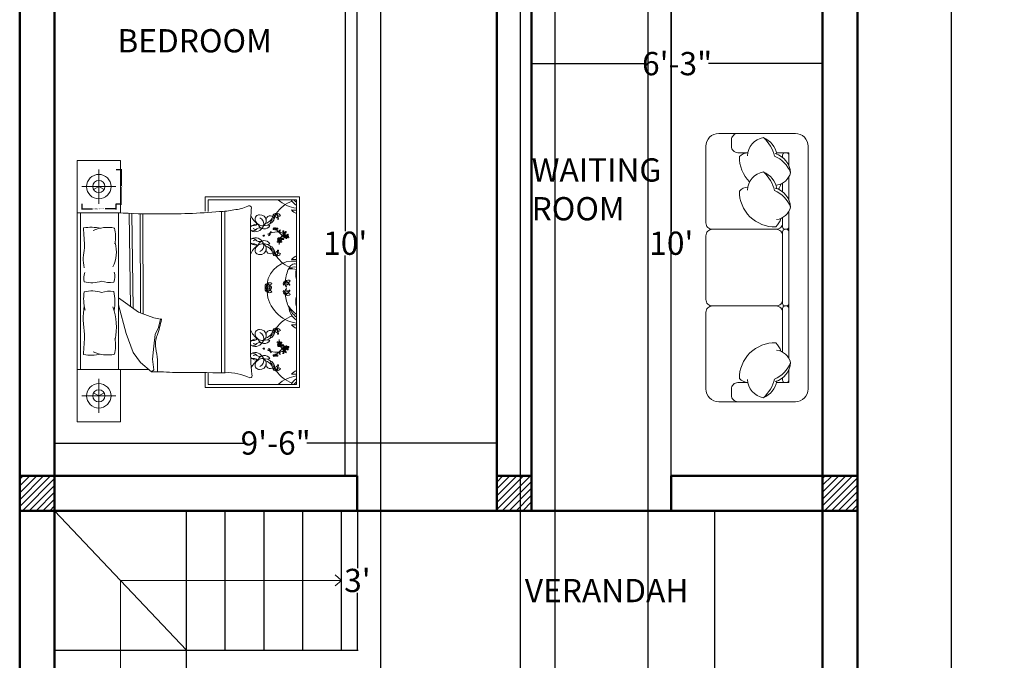
# Model space of a CAD drawing. Units: inches. Extents: x 0 to 281, y -535 to 46.
# Tile 2 of 22: x 27 to 281, y -440 to -275. Entities that reach past the tile are written whole.
import ezdxf

# ---------------------------------------------------------------- set-up
doc = ezdxf.new("R2010")
doc.units = ezdxf.units.IN
doc.header["$MEASUREMENT"] = 0
for name, color, linetype, lineweight in [('A-ANNO-DIMS', 2, 'Continuous', 18), ('A-ANNO-SYMB', 2, 'Continuous', 18), ('A-AREA-IDEN', 7, 'Continuous', 25), ('A-COLS', 7, 'Continuous', 50), ('A-COLS-PATT', 152, 'Continuous', 13), ('A-FLOR-STRS', 7, 'Continuous', 25), ('A-FURN', 8, 'Continuous', 18), ('A-WALL', 7, 'Continuous', 50)]:
    doc.layers.add(name, color=color, linetype=linetype, lineweight=lineweight)
doc.styles.get("Standard").update_dxf_attribs({"font": 'arial.ttf'})
doc.dimstyles.get("Standard").update_dxf_attribs({"dimtxt": 0.18, "dimasz": 0.18, "dimexe": 0.18, "dimexo": 0.0625, "dimgap": 0.09, "dimtad": 0, "dimtih": 1, "dimtoh": 1, "dimdec": 0, "dimzin": 0, "dimdsep": 46, "dimlunit": 3, "dimtxsty": 'Standard', "dimcen": 0.09, "dimadec": 0, "dimazin": 0, "dimtfac": 1, "dimtdec": 0, "dimtofl": 0, "dimtmove": 0, "dimatfit": 3, "dimfxl": 1, "dimtolj": 1, "dimtzin": 0, "dimarcsym": 0})

# ---------------------------------------------------------------- blocks, each defined once
blk = doc.blocks.new('*D9')
at = {"layer": 'A-ANNO-DIMS', "color": 0, "lineweight": -2, "transparency": 16777216}
for p, q in [((114.4, -272.41), (111.21, -272.41)), ((111.39, -272.59), (111.39, -329.26)), ((111.39, -392.23), (111.39, -335.56)), ((114.4, -392.41), (111.21, -392.41))]:
    blk.add_line(p, q, dxfattribs=at)
at = {"layer": 'A-ANNO-DIMS', "color": 0, "transparency": 16777216}
for points in [[(111.36, -272.59), (111.42, -272.59), (111.39, -272.41)], [(111.36, -392.23), (111.42, -392.23), (111.39, -392.41)]]:
    blk.add_solid(points, dxfattribs=at)
at = {"layer": 'Defpoints', "color": 0, "transparency": 16777216}
for p in [(111.39, -272.41), (114.46, -272.41), (114.46, -392.41)]:
    blk.add_point(p, dxfattribs=at)
at = {"layer": 'A-ANNO-DIMS', "color": 0, "transparency": 16777216, "insert": (111.39, -332.41), "char_height": 6, "attachment_point": 5}
blk.add_mtext("\\A1;10'", dxfattribs=at)
blk = doc.blocks.new('*D10')
at = {"layer": 'A-ANNO-DIMS', "color": 0, "lineweight": -2, "transparency": 16777216}
for p, q in [((36.46, -383.89), (36.46, -383.77)), ((36.64, -383.95), (85.39, -383.95)), ((150.28, -383.95), (101.52, -383.95)), ((150.46, -383.89), (150.46, -383.77))]:
    blk.add_line(p, q, dxfattribs=at)
at = {"layer": 'A-ANNO-DIMS', "color": 0, "transparency": 16777216}
for points in [[(36.64, -383.92), (36.64, -383.98), (36.46, -383.95)], [(150.28, -383.92), (150.28, -383.98), (150.46, -383.95)]]:
    blk.add_solid(points, dxfattribs=at)
at = {"layer": 'Defpoints', "color": 0, "transparency": 16777216}
for p in [(36.46, -383.95), (150.46, -383.95), (150.46, -383.95)]:
    blk.add_point(p, dxfattribs=at)
at = {"layer": 'A-ANNO-DIMS', "color": 0, "transparency": 16777216, "insert": (93.46, -383.95), "char_height": 6, "attachment_point": 5}
blk.add_mtext('\\A1;9\'-6"', dxfattribs=at)
blk = doc.blocks.new('*D11')
at = {"layer": 'A-ANNO-DIMS', "color": 0, "lineweight": -2, "transparency": 16777216}
for p, q in [((159.46, -286.02), (159.46, -285.9)), ((159.64, -286.08), (188.88, -286.08)), ((234.28, -286.08), (205.04, -286.08)), ((234.46, -286.02), (234.46, -285.9))]:
    blk.add_line(p, q, dxfattribs=at)
at = {"layer": 'A-ANNO-DIMS', "color": 0, "transparency": 16777216}
for points in [[(159.64, -286.05), (159.64, -286.11), (159.46, -286.08)], [(234.28, -286.05), (234.28, -286.11), (234.46, -286.08)]]:
    blk.add_solid(points, dxfattribs=at)
at = {"layer": 'Defpoints', "color": 0, "transparency": 16777216}
for p in [(159.46, -286.08), (234.46, -286.08), (234.46, -286.08)]:
    blk.add_point(p, dxfattribs=at)
at = {"layer": 'A-ANNO-DIMS', "color": 0, "transparency": 16777216, "insert": (196.96, -286.08), "char_height": 6, "attachment_point": 5}
blk.add_mtext('\\A1;6\'-3"', dxfattribs=at)
blk = doc.blocks.new('*D12')
at = {"layer": 'A-ANNO-DIMS', "color": 0, "lineweight": -2, "transparency": 16777216}
for p, q in [((195.46, -272.59), (195.46, -329.26)), ((195.52, -272.41), (195.64, -272.41)), ((195.46, -392.23), (195.46, -335.56)), ((195.52, -392.41), (195.64, -392.41))]:
    blk.add_line(p, q, dxfattribs=at)
at = {"layer": 'A-ANNO-DIMS', "color": 0, "transparency": 16777216}
for points in [[(195.43, -272.59), (195.49, -272.59), (195.46, -272.41)], [(195.43, -392.23), (195.49, -392.23), (195.46, -392.41)]]:
    blk.add_solid(points, dxfattribs=at)
at = {"layer": 'Defpoints', "color": 0, "transparency": 16777216}
for p in [(195.46, -272.41), (195.46, -392.41), (195.46, -392.41)]:
    blk.add_point(p, dxfattribs=at)
at = {"layer": 'A-ANNO-DIMS', "color": 0, "transparency": 16777216, "insert": (195.46, -332.41), "char_height": 6, "attachment_point": 5}
blk.add_mtext("\\A1;10'", dxfattribs=at)
blk = doc.blocks.new('*D13')
at = {"layer": 'A-ANNO-DIMS', "color": 0, "lineweight": -2, "transparency": 16777216}
for p, q in [((206.57, -401.59), (206.57, -446.76)), ((206.63, -401.41), (206.75, -401.41)), ((206.57, -498.23), (206.57, -453.06)), ((206.63, -498.41), (206.75, -498.41))]:
    blk.add_line(p, q, dxfattribs=at)
at = {"layer": 'A-ANNO-DIMS', "color": 0, "transparency": 16777216}
for points in [[(206.54, -401.59), (206.6, -401.59), (206.57, -401.41)], [(206.54, -498.23), (206.6, -498.23), (206.57, -498.41)]]:
    blk.add_solid(points, dxfattribs=at)
at = {"layer": 'Defpoints', "color": 0, "transparency": 16777216}
for p in [(206.57, -401.41), (206.57, -498.41), (206.57, -498.41)]:
    blk.add_point(p, dxfattribs=at)
at = {"layer": 'A-ANNO-DIMS', "color": 0, "transparency": 16777216, "insert": (206.57, -449.91), "char_height": 6, "attachment_point": 5}
blk.add_mtext('\\A1;8\'-1"', dxfattribs=at)
blk = doc.blocks.new('*D15')
at = {"layer": 'A-ANNO-DIMS', "color": 0, "lineweight": -2, "transparency": 16777216}
for p, q in [((110.52, -401.41), (114.71, -401.41)), ((114.53, -401.59), (114.53, -416.26)), ((114.53, -437.23), (114.53, -422.57)), ((110.52, -437.41), (114.71, -437.41))]:
    blk.add_line(p, q, dxfattribs=at)
at = {"layer": 'A-ANNO-DIMS', "color": 0, "transparency": 16777216}
for points in [[(114.5, -401.59), (114.56, -401.59), (114.53, -401.41)], [(114.5, -437.23), (114.56, -437.23), (114.53, -437.41)]]:
    blk.add_solid(points, dxfattribs=at)
at = {"layer": 'Defpoints', "color": 0, "transparency": 16777216}
for p in [(110.46, -401.41), (110.46, -437.41), (114.53, -437.41)]:
    blk.add_point(p, dxfattribs=at)
at = {"layer": 'A-ANNO-DIMS', "color": 0, "transparency": 16777216, "insert": (114.53, -419.41), "char_height": 6, "attachment_point": 5}
blk.add_mtext("\\A1;3'", dxfattribs=at)
blk = doc.blocks.new('*D18')
at = {"layer": 'A-ANNO-DIMS', "color": 0, "lineweight": -2, "transparency": 16777216}
for p, q in [((243.52, 18.59), (267.93, 18.59)), ((267.75, 18.41), (267.75, -241.26)), ((267.75, -507.23), (267.75, -247.57)), ((243.52, -507.41), (267.93, -507.41))]:
    blk.add_line(p, q, dxfattribs=at)
at = {"layer": 'A-ANNO-DIMS', "color": 0, "transparency": 16777216}
for points in [[(267.72, 18.41), (267.78, 18.41), (267.75, 18.59)], [(267.72, -507.23), (267.78, -507.23), (267.75, -507.41)]]:
    blk.add_solid(points, dxfattribs=at)
at = {"layer": 'Defpoints', "color": 0, "transparency": 16777216}
for p in [(243.46, 18.59), (243.46, -507.41), (267.75, -507.41)]:
    blk.add_point(p, dxfattribs=at)
at = {"layer": 'A-ANNO-DIMS', "color": 0, "transparency": 16777216, "insert": (267.75, -244.41), "char_height": 6, "attachment_point": 5}
blk.add_mtext('\\A1;43\'-10"', dxfattribs=at)
blk = doc.blocks.new('BEDSIDE-LAMP-SMALL')
for p, q in [((4.41, 0), (4.41, 8.82)), ((8.82, 4.41), (0, 4.41))]:
    blk.add_line(p, q)
for points in [[(4.41, 4.41), (3.04, 3.62)], [(4.41, 4.41), (5.77, 3.62)]]:
    blk.add_lwpolyline(points)
for radius in [3.15, 1.57]:
    blk.add_circle((4.41, 4.41), radius)
blk = doc.blocks.new('SOFA-THROW-PILLOW')
for points in [[(11.04, 3.89, 0.165541), (13.21, 4.91, 0.425989), (3.78, 14.16, 0.121523), (2.47, 11.97, -7.115464)], [(3.93, 4.15, -0.306663), (0, 9.06, -0.30633), (3.59, 12.27, 0.872847)], [(6.98, 0, -0.14773), (4.15, 4.82, -0.213343), (0, 9.06, -0.178662)], [(11.14, 4.72, -0.356772), (6.98, 0, -0.249542), (3.56, 4.28, 9.61688)]]:
    blk.add_lwpolyline(points, format="xyb")
blk = doc.blocks.new('*D38')
at = {"layer": 'A-ANNO-DIMS', "color": 0, "lineweight": -2, "transparency": 16777216}
for p, q in [((43.45, -322.28), (43.45, -323.72)), ((52.27, -322.28), (52.27, -323.72)), ((43.63, -323.54), (46.26, -323.54)), ((52.09, -323.54), (49.46, -323.54))]:
    blk.add_line(p, q, dxfattribs=at)
at = {"layer": 'A-ANNO-DIMS', "color": 0, "transparency": 16777216}
for points in [[(43.63, -323.51), (43.63, -323.57), (43.45, -323.54)], [(52.09, -323.51), (52.09, -323.57), (52.27, -323.54)]]:
    blk.add_solid(points, dxfattribs=at)
at = {"layer": 'Defpoints', "color": 0, "transparency": 16777216}
for p in [(43.45, -322.21), (52.27, -322.21), (52.27, -323.54)]:
    blk.add_point(p, dxfattribs=at)
at = {"layer": 'A-ANNO-DIMS', "color": 0, "transparency": 16777216, "insert": (47.86, -323.54), "char_height": 0.18, "attachment_point": 5}
blk.add_mtext('\\A1;BEDSIDE LAMP 0\'-9" TYP.', dxfattribs=at)
blk = doc.blocks.new('*D39')
at = {"layer": 'A-ANNO-DIMS', "color": 0, "lineweight": -2, "transparency": 16777216}
for p, q in [((52.33, -313.4), (53.77, -313.4)), ((53.59, -313.58), (53.59, -317.63)), ((53.59, -322.03), (53.59, -317.99)), ((52.33, -322.21), (53.77, -322.21))]:
    blk.add_line(p, q, dxfattribs=at)
at = {"layer": 'A-ANNO-DIMS', "color": 0, "transparency": 16777216}
for points in [[(53.56, -313.58), (53.62, -313.58), (53.59, -313.4)], [(53.56, -322.03), (53.62, -322.03), (53.59, -322.21)]]:
    blk.add_solid(points, dxfattribs=at)
at = {"layer": 'Defpoints', "color": 0, "transparency": 16777216}
for p in [(52.27, -313.4), (53.59, -313.4), (52.27, -322.21)]:
    blk.add_point(p, dxfattribs=at)
at = {"layer": 'A-ANNO-DIMS', "color": 0, "transparency": 16777216, "insert": (53.59, -317.81), "char_height": 0.18, "attachment_point": 5}
blk.add_mtext('\\A1;0\'-9" TYP.', dxfattribs=at)
blk = doc.blocks.new('*D41')
at = {"layer": 'A-ANNO-DIMS', "color": 0, "lineweight": -2, "transparency": 16777216}
for p, q in [((120.46, -131.47), (120.46, -535.04)), ((156.46, -131.47), (156.46, -535.04)), ((120.64, -534.86), (138.13, -534.86)), ((156.28, -534.86), (138.79, -534.86))]:
    blk.add_line(p, q, dxfattribs=at)
at = {"layer": 'A-ANNO-DIMS', "color": 0, "transparency": 16777216}
for points in [[(120.64, -534.83), (120.64, -534.89), (120.46, -534.86)], [(156.28, -534.83), (156.28, -534.89), (156.46, -534.86)]]:
    blk.add_solid(points, dxfattribs=at)
at = {"layer": 'Defpoints', "color": 0, "transparency": 16777216}
for p in [(120.46, -131.41), (156.46, -131.41), (156.46, -534.86)]:
    blk.add_point(p, dxfattribs=at)
at = {"layer": 'A-ANNO-DIMS', "color": 0, "transparency": 16777216, "insert": (138.46, -534.86), "char_height": 0.18, "attachment_point": 5}
blk.add_mtext('\\A1;3\'-0"', dxfattribs=at)
blk = doc.blocks.new('*D42')
at = {"layer": 'A-ANNO-DIMS', "color": 0, "lineweight": -2, "transparency": 16777216}
for p, q in [((165.46, -131.47), (165.46, -535.04)), ((189.46, -131.47), (189.46, -535.04)), ((165.64, -534.86), (177.13, -534.86)), ((189.28, -534.86), (177.79, -534.86))]:
    blk.add_line(p, q, dxfattribs=at)
at = {"layer": 'A-ANNO-DIMS', "color": 0, "transparency": 16777216}
for points in [[(165.64, -534.83), (165.64, -534.89), (165.46, -534.86)], [(189.28, -534.83), (189.28, -534.89), (189.46, -534.86)]]:
    blk.add_solid(points, dxfattribs=at)
at = {"layer": 'Defpoints', "color": 0, "transparency": 16777216}
for p in [(165.46, -131.41), (189.46, -131.41), (189.46, -534.86)]:
    blk.add_point(p, dxfattribs=at)
at = {"layer": 'A-ANNO-DIMS', "color": 0, "transparency": 16777216, "insert": (177.46, -534.86), "char_height": 0.18, "attachment_point": 5}
blk.add_mtext('\\A1;2\'-0"', dxfattribs=at)
blk = doc.blocks.new('*D47')
at = {"layer": 'A-ANNO-DIMS', "color": 0, "lineweight": -2, "transparency": 16777216}
for p, q in [((114.46, -392.35), (114.46, 46.22)), ((114.64, 46.04), (132.13, 46.04)), ((150.28, 46.04), (132.79, 46.04)), ((150.46, -392.35), (150.46, 46.22))]:
    blk.add_line(p, q, dxfattribs=at)
at = {"layer": 'A-ANNO-DIMS', "color": 0, "transparency": 16777216}
for points in [[(114.64, 46.07), (114.64, 46.01), (114.46, 46.04)], [(150.28, 46.07), (150.28, 46.01), (150.46, 46.04)]]:
    blk.add_solid(points, dxfattribs=at)
at = {"layer": 'Defpoints', "color": 0, "transparency": 16777216}
for p in [(150.46, 46.04), (114.46, -392.41), (150.46, -392.41)]:
    blk.add_point(p, dxfattribs=at)
at = {"layer": 'A-ANNO-DIMS', "color": 0, "transparency": 16777216, "insert": (132.46, 46.04), "char_height": 0.18, "attachment_point": 5}
blk.add_mtext('\\A1;3\'-0"', dxfattribs=at)
blk = doc.blocks.new('*D48')
at = {"layer": 'A-ANNO-DIMS', "color": 0, "lineweight": -2, "transparency": 16777216}
for p, q in [((159.46, -392.35), (159.46, 46.22)), ((159.64, 46.04), (177.13, 46.04)), ((195.28, 46.04), (177.79, 46.04)), ((195.46, -392.35), (195.46, 46.22))]:
    blk.add_line(p, q, dxfattribs=at)
at = {"layer": 'A-ANNO-DIMS', "color": 0, "transparency": 16777216}
for points in [[(159.64, 46.07), (159.64, 46.01), (159.46, 46.04)], [(195.28, 46.07), (195.28, 46.01), (195.46, 46.04)]]:
    blk.add_solid(points, dxfattribs=at)
at = {"layer": 'Defpoints', "color": 0, "transparency": 16777216}
for p in [(195.46, 46.04), (159.46, -392.41), (195.46, -392.41)]:
    blk.add_point(p, dxfattribs=at)
at = {"layer": 'A-ANNO-DIMS', "color": 0, "transparency": 16777216, "insert": (177.46, 46.04), "char_height": 0.18, "attachment_point": 5}
blk.add_mtext('\\A1;3\'-0"', dxfattribs=at)

msp = doc.modelspace()

# ---------------------------------------------------------------- hatches: boundary and pattern name
at = {"layer": 'A-COLS-PATT'}
h = msp.add_hatch(dxfattribs=at)
h.set_pattern_fill('ANSI31', color=256, scale=10)
h.paths.add_polyline_path([(36.46, 18.59), (27.46, 18.59), (27.46, 9.59), (36.46, 9.59)])
h.paths.add_polyline_path([(165.46, 18.59), (156.46, 18.59), (156.46, 9.59), (165.46, 9.59)])
h.paths.add_polyline_path([(243.46, 18.59), (234.46, 18.59), (234.46, 9.59), (243.46, 9.59)])
h.paths.add_polyline_path([(243.46, -122.41), (234.46, -122.41), (234.46, -131.41), (243.46, -131.41)])
h.paths.add_polyline_path([(36.46, -122.41), (27.46, -122.41), (27.46, -131.41), (36.46, -131.41)])
h.paths.add_polyline_path([(36.46, -498.41), (27.46, -498.41), (27.46, -507.41), (36.46, -507.41)])
h.paths.add_polyline_path([(243.46, -498.41), (234.46, -498.41), (234.46, -507.41), (243.46, -507.41)])
h.paths.add_polyline_path([(159.46, -498.41), (150.46, -498.41), (150.46, -507.41), (159.46, -507.41)])
h.paths.add_polyline_path([(36.46, -392.41), (27.46, -392.41), (27.46, -401.41), (36.46, -401.41)])
h.paths.add_polyline_path([(159.46, -392.41), (150.46, -392.41), (150.46, -401.41), (159.46, -401.41)])
h.paths.add_polyline_path([(243.46, -392.41), (234.46, -392.41), (234.46, -401.41), (243.46, -401.41)])
h.paths.add_polyline_path([(36.46, -263.41), (27.46, -263.41), (27.46, -272.41), (36.46, -272.41)])
h.paths.add_polyline_path([(243.46, -263.41), (234.46, -263.41), (234.46, -272.41), (243.46, -272.41)])

# ---------------------------------------------------------------- linework, layer by layer
at = {"layer": 'A-ANNO-SYMB'}
for p, q in [((110.46, -419.41), (108.77, -418)), ((110.46, -419.41), (53.46, -419.41)), ((53.46, -419.41), (53.46, -480.41)), ((110.46, -419.41), (108.77, -420.82))]:
    msp.add_line(p, q, dxfattribs=at)
at = {"layer": 'A-COLS'}
msp.add_line((150.46, -392.41), (159.46, -392.41), dxfattribs=at)
at = {"layer": 'A-FLOR-STRS'}
for p, q in [((70.46, -437.41), (36.46, -401.41)), ((70.46, -498.41), (70.46, -401.41)), ((80.46, -437.41), (80.46, -401.41)), ((90.46, -437.41), (90.46, -401.41)), ((100.46, -437.41), (100.46, -401.41)), ((110.46, -437.41), (110.46, -401.41)), ((36.46, -437.41), (110.46, -437.41))]:
    msp.add_line(p, q, dxfattribs=at)
at = {"layer": 'A-FURN'}
for p, q in [((42.24, -378.52), (42.24, -311.06)), ((75.31, -324.18), (75.31, -320.44)), ((75.31, -320.44), (99.61, -320.44)), ((76.09, -321.22), (76.09, -324.19)), ((98.83, -321.22), (76.09, -321.22)), ((98.83, -368.84), (98.83, -321.22)), ((99.61, -320.44), (99.61, -369.62)), ((43.11, -324.55), (43.11, -365.03)), ((52.9, -365.03), (52.9, -324.55)), ((55.7, -324.73), (56.04, -348.75)), ((56.39, -324.76), (56.74, -349.26)), ((58.52, -324.8), (58.62, -350.41)), ((59.21, -324.79), (59.32, -350.68)), ((79.52, -324.25), (79.52, -365.81)), ((80.36, -324.18), (80.36, -365.81)), ((91.99, -327.87), (91.23, -327.72)), ((86.98, -331.1), (86.98, -358.49)), ((91.99, -332.58), (91.23, -332.73)), ((52.9, -346.5), (58.05, -350.19)), ((54.9, -355.66), (52.9, -348.3)), ((58.05, -350.19), (62.01, -351.7)), ((62.01, -351.7), (63.78, -351.97)), ((63.78, -351.97), (63.23, -354.16)), ((63.23, -354.16), (62.41, -355.93)), ((56.68, -360.58), (54.9, -355.66)), ((62.41, -355.93), (62.01, -358.94)), ((91.99, -357.47), (91.23, -357.32)), ((62.01, -358.94), (61.73, -362.35)), ((58.59, -363.17), (56.68, -360.58)), ((61.73, -362.35), (62.01, -365.09)), ((91.99, -362.19), (91.23, -362.34)), ((42.24, -365.03), (60.75, -365.03)), ((61.46, -365.63), (58.59, -363.17)), ((62.01, -365.09), (61.46, -365.63)), ((75.31, -369.62), (75.31, -365.8)), ((76.09, -365.8), (76.09, -368.84)), ((99.61, -369.62), (75.31, -369.62)), ((76.09, -368.84), (98.83, -368.84))]:
    msp.add_line(p, q, dxfattribs=at)
at = {"layer": 'A-FURN', "ltscale": 0.03}
msp.add_lwpolyline([(207.69, -373.3, -0.414214), (204.39, -370.01), (204.39, -350.24, -0.414214), (206.04, -348.59, -0.414214), (204.39, -346.94), (204.39, -330.47, -0.414214), (206.04, -328.82, -0.414214), (204.39, -327.17), (204.39, -307.4, -0.414214), (207.69, -304.11), (227.46, -304.11, -0.414214), (230.75, -307.4), (230.75, -370.01, -0.414214), (227.46, -373.3)], format="xyb", close=True, dxfattribs=at)
at = {"layer": 'A-FURN'}
for points in [[(215.18, -309.05), (212.63, -309.05, -0.414214), (210.98, -307.4), (210.98, -305.75, -0.414214), (212.63, -304.11)], [(215.08, -309.88, -0.356772), (219.24, -305.15, -0.249542), (222.66, -309.43, 9.61688)], [(219.24, -305.15, -0.14773), (222.07, -309.97, -0.213343), (226.22, -314.22, -0.178662)], [(215.18, -309.05, 0.165541), (213.01, -310.06, 0.200231), (215.66, -316.6, 0.121523)], [(222.29, -309.3, -0.306663), (226.22, -314.22, -0.30633), (222.63, -317.43, 0.872847)], [(225.81, -312.51), (225.81, -309.05), (222.57, -309.05, -0.414214)], [(224.16, -310.31), (224.16, -309.71, -0.414214), (224.82, -309.05), (225.15, -309.05, -0.414214), (225.81, -309.71)], [(225.81, -309.71), (225.81, -312.51, -0.414214)], [(223.1, -318.5, 0.071865), (223.75, -317.12, -7.115464)], [(224.16, -319.18), (224.16, -316.91, -0.414214)], [(225.81, -315.26), (225.81, -321.39, -0.414214)], [(78.98, -324.27, 0.056112), (82.7, -323.78, 0.095341), (86.27, -322.83)], [(225.81, -324.13), (225.81, -328.16, -0.414214), (225.15, -328.82), (224.82, -328.82, -0.414214), (224.16, -328.16), (224.16, -325.79, -0.414214)], [(224.16, -327.17, -0.414214), (222.52, -328.82), (206.04, -328.82, -0.414214)], [(43.92, -328.43, -0.074897), (48.33, -328.51, 0.472817)], [(224.16, -330.47, 0.414214), (222.52, -328.82)], [(48.57, -342.23, -0.14099), (44.08, -342.36, -0.235245)], [(48.57, -345.11, 0.14099), (44.08, -344.97, 0.235245)], [(224.16, -346.94, -0.414214), (222.52, -348.59)], [(224.16, -350.24, 0.414214), (222.52, -348.59), (206.04, -348.59, 0.414214)], [(225.81, -362.15), (225.81, -349.25, 0.414214), (225.15, -348.59), (224.82, -348.59, 0.414214), (224.16, -349.25), (224.16, -360.5, 0.414214)], [(43.92, -361.15, 0.074897), (48.33, -361.07, -0.472817)], [(225.81, -367.7), (225.81, -364.9, 0.414214)], [(67.64, -365.77, 0.001242), (80.44, -365.81, -0.127202), (86.81, -367.16)], [(224.16, -367.1), (224.16, -367.7, 0.414214), (224.82, -368.36), (225.15, -368.36, 0.414214), (225.81, -367.7)], [(212.63, -373.3, -0.414214), (210.98, -371.66), (210.98, -370.01, -0.414214), (212.63, -368.36), (215.18, -368.36)]]:
    msp.add_lwpolyline(points, format="xyb", dxfattribs=at)
for points in [[(42.24, -324.55), (53.48, -324.55), (53.48, -311.06), (42.24, -311.06)], [(225.81, -321.39), (225.81, -315.26)], [(225.81, -362.15), (225.81, -324.13)], [(53.48, -365.03), (53.48, -378.52), (42.24, -378.52)], [(222.57, -368.36), (225.81, -368.36), (225.81, -364.9)]]:
    msp.add_lwpolyline(points, dxfattribs=at)
msp.add_lwpolyline([(225.81, -329.48), (225.81, -347.93, -0.414214), (225.15, -348.59), (224.82, -348.59, -0.414214), (224.16, -347.93), (224.16, -329.48, -0.414214), (224.82, -328.82), (225.15, -328.82, -0.414214)], format="xyb", close=True, dxfattribs=at)
for centre in [(94.43, -331.76), (96.24, -330.64), (94.43, -358.29), (96.24, -359.41)]:
    msp.add_circle(centre, 0.172, dxfattribs=at)
for centre, radius, start, end in [((100.89, -329.73), 8.81, 111.4092, 145.6135), ((100.01, -314.66), 8.81, 228.1144, 262.255), ((101.19, -319.08), 4.29, 209.8884, 236.5383), ((101.99, -317.53), 5.35, 223.5186, 233.6964), ((61.14, -203.62), 121.21, 266.1, 270.9282), ((65.55, -166.72), 158.12, 269.1145, 274.8735), ((86.61, -323.34), 0.615, 336.5219, 123.8264), ((152.59, -329.03), 65.64, 175.2402, 181.8035), ((93.44, -325.46), 0.73, 76.272, 177.0484), ((92.33, -323.97), 1.5, 284.7031, 328.6173), ((94.43, -325.89), 1.39, 125.7657, 194.5347), ((87.6, -323.42), 6.16, 332.8176, 347.4827), ((93.82, -325.71), 0.977, 20.9613, 102.2885), ((94.35, -324.73), 0.736, 181.7131, 301.5367), ((91.94, -326.22), 2.23, 2.0648, 41.1598), ((93.28, -325.39), 0.721, 316.2238, 62.3173), ((100.2, -321.48), 3.58, 221.0454, 247.4453), ((98.28, -311.67), 12.19, 266.3481, 272.5919), ((91.73, -323.25), 5.11, 203.6453, 236.3329), ((88.7, -330.09), 2.6, 85.2696, 124.215), ((89.28, -326.23), 1.14, 88.9462, 185.5144), ((90.13, -325.88), 2.03, 193.079, 274.7067), ((89.45, -326.69), 1.61, 7.1143, 95.0551), ((88.83, -327.33), 1.57, 338.5779, 68.4181), ((89.09, -326.41), 1.96, 305.9599, 357.6409), ((90.07, -324.29), 3.62, 273.4924, 303.7117), ((89.81, -324.32), 3.18, 288.2955, 328.7386), ((92.04, -326.32), 1.01, 19.1312, 189.736), ((91.74, -326.08), 1.26, 285.6955, 4.031), ((93.42, -327.44), 1.35, 128.4175, 173.8338), ((93.14, -326.11), 0.621, 126.7319, 206.0245), ((93.7, -325.82), 0.0574, 20.2667, 316.2271), ((94, -326.13), 0.0531, 52.0591, 168.5166), ((94.06, -326.15), 0.109, 168.5166, 2.0648), ((-598.08, -365.61), 643.07, 2.85022, 3.31479), ((50.1, -337.02), 8.69, 78.2417, 114.8684), ((43.13, -330.83), 9.04, 348.9631, 14.8961), ((87.73, -328.59), 0.812, 127.675, 162.5814), ((87.73, -328.59), 0.812, 196.6343, 225.5483), ((87.48, -325.12), 2.79, 259.249, 301.1782), ((88.21, -327.29), 2.15, 240.8249, 340.7178), ((87.57, -328.24), 1.01, 246.1646, 318.4347), ((88.6, -326.96), 1.94, 240.0851, 262.564), ((89.36, -329.83), 1.38, 74.8529, 138.4347), ((90.53, -327.03), 1.68, 196.8663, 330.0915), ((89.83, -328.09), 0.419, 254.8529, 12.6959), ((88.7, -330.09), 2.6, 53.6555, 57.2989), ((93.86, -335.09), 5.59, 110.1059, 116.9968), ((91.95, -330.06), 0.137, 83.9457, 185.6216), ((91.4, -329.93), 0.565, 328.836, 0.8141), ((91.69, -330.09), 0.324, 306.5232, 32.4668), ((92.08, -329.84), 0.137, 112.5583, 214.2343), ((91.99, -329.6), 0.324, 265.7131, 351.6568), ((91.7, -329.42), 0.565, 297.3659, 329.344), ((91.28, -328.93), 1.08, 313.6929, 321.7899), ((92.47, -329.67), 0.354, 115.5379, 168.6744), ((91.27, -329.16), 1.07, 329.344, 349.7412), ((93.86, -335.09), 5.59, 86.1723, 106.4158), ((90.42, -329.41), 1.9, 352.8698, 1.6736), ((92.94, -328.72), 0.133, 125.0752, 284.7644), ((93.15, -328.67), 0.287, 127.3642, 168.4363), ((92.92, -328.44), 0.413, 277.4968, 341.2737), ((93.25, -328.63), 0.164, 88.1325, 178.8919), ((93.58, -328.81), 0.355, 136.3462, 189.6513), ((93.37, -328.84), 0.148, 189.6513, 312.3208), ((93.41, -328.43), 0.172, 183.2768, 356.7232), ((93.95, -328.74), 0.562, 164.2829, 186.9148), ((93.29, -328.74), 0.281, 312.3208, 40.2111), ((93.88, -328.43), 0.399, 201.6382, 274.947), ((93.35, -328.97), 0.522, 42.3896, 66.5724), ((98.61, -324.84), 6.41, 217.9541, 226.8459), ((93.73, -328.67), 0.284, 10.9597, 52.2379), ((93.9, -328.69), 0.132, 274.947, 37.5263), ((94.35, -329.44), 0.137, 112.5583, 214.2343), ((94.26, -329.19), 0.324, 265.7131, 351.6568), ((93.97, -329.02), 0.565, 297.3659, 329.344), ((94, -332.31), 2.8, 60.7959, 85.244), ((88.04, -336.34), 9.22, 37.8256, 47.7588), ((93.55, -328.53), 1.08, 313.6929, 321.7899), ((94.74, -329.27), 0.354, 115.5379, 168.6744), ((93.54, -328.76), 1.07, 329.344, 349.7412), ((92.69, -329.01), 1.9, 352.8698, 1.6736), ((97.72, -332.6), 3.36, 130.182, 149.456), ((95.37, -329.39), 0.192, 33.0979, 123.1364), ((91.14, -332.09), 5.02, 31.1156, 34.8118), ((95.09, -329.72), 0.519, 2.3172, 70.5201), ((94.84, -330.28), 0.783, 310.9365, 22.7695), ((95.52, -329.85), 0.15, 135.7354, 318.1297), ((95.27, -329.6), 0.199, 315.7354, 31.1156), ((95.1, -330.02), 0.461, 319.3812, 5.5456), ((95.63, -329.85), 0.15, 68.2452, 250.6395), ((95.28, -329.66), 0.447, 352.6008, 57.1845), ((96.88, -332.66), 2.99, 111.7087, 116.2181), ((94, -332.31), 2.8, 47.5083, 55.9967), ((95.71, -329.56), 0.447, 252.8042, 349.6943), ((95.28, -330.36), 0.476, 331.1838, 51.6792), ((95.76, -329.52), 0.199, 248.2452, 323.6254), ((95.58, -329.4), 0.519, 291.7087, 3.0299), ((91.88, -326.66), 5.02, 323.6254, 327.3216), ((95.99, -329.53), 0.192, 325.6077, 55.6462), ((43.8, -334.74), 8.59, 333.8761, 16.1746), ((87.73, -331.86), 0.812, 134.4517, 156.7144), ((87.73, -331.86), 0.812, 203.2856, 232.325), ((87.48, -335.32), 2.79, 58.8218, 100.2867), ((88.21, -333.16), 2.15, 19.2822, 119.1751), ((87.57, -332.2), 1.01, 41.5653, 113.8354), ((88.7, -330.35), 2.6, 235.785, 274.7304), ((88.6, -333.48), 1.94, 97.436, 119.9149), ((90.13, -334.57), 2.03, 85.2933, 166.921), ((89.36, -330.62), 1.38, 221.5653, 285.1471), ((90.53, -333.42), 1.68, 29.9085, 163.1337), ((88.83, -333.12), 1.57, 291.5819, 21.4221), ((89.83, -332.35), 0.419, 347.3041, 105.1471), ((88.7, -330.35), 2.6, 302.7011, 306.3445), ((90.38, -330.4), 0.211, 169.5864, 349.5616), ((89.09, -334.03), 1.96, 2.3591, 54.0401), ((90.07, -336.16), 3.62, 56.2883, 86.5076), ((90.46, -330.42), 0.13, 349.5616, 167.2949), ((91.99, -330.49), 0.354, 129.5056, 182.6421), ((90.97, -329.67), 1.07, 308.4388, 328.836), ((90.78, -328.8), 1.9, 296.5064, 305.3102), ((90.77, -329.78), 1.08, 336.3901, 344.4871), ((93.96, -332.05), 0.133, 125.0752, 284.7644), ((94.17, -332), 0.287, 93.635, 168.4363), ((94.18, -330.45), 0.783, 253.6301, 325.4631), ((94.4, -331.53), 0.554, 82.0748, 142.6895), ((94.33, -330.77), 0.569, 228.342, 274.9894), ((94.13, -331.55), 0.168, 138.2946, 276.2474), ((94.19, -331.57), 0.234, 358.5719, 143.8954), ((93.94, -331.77), 0.413, 277.4968, 341.2737), ((94.27, -331.96), 0.164, 88.1325, 178.8919), ((94.33, -331.39), 0.236, 208.8493, 269.9355), ((94.13, -331.45), 0.27, 274.2123, 318.1587), ((94.6, -332.14), 0.355, 136.3462, 189.6513), ((94.4, -332.17), 0.148, 189.6513, 312.3208), ((97.72, -332.6), 3.36, 175.2415, 182.8929), ((94.35, -330.87), 0.476, 273.8774, 357.1501), ((94.97, -332.07), 0.562, 164.2829, 186.9148), ((94.95, -331.72), 0.542, 121.9501, 165.2442), ((94.54, -330.53), 0.461, 262.0748, 308.2393), ((94.31, -332.07), 0.281, 312.3208, 40.2111), ((94.9, -331.76), 0.399, 201.6382, 274.947), ((94.58, -331.51), 0.114, 262.868, 7.094), ((94.37, -332.3), 0.522, 42.3896, 66.5724), ((94.56, -331.41), 0.339, 278.5614, 22.5914), ((94.75, -332), 0.284, 10.9597, 118.7804), ((97.72, -332.6), 3.36, 156.1523, 156.9499), ((94.76, -331.4), 0.17, 44.3732, 121.9501), ((95.28, -331), 0.476, 181.4625, 249.4747), ((95.2, -330.63), 0.461, 215.1128, 261.2773), ((95.57, -330.65), 0.783, 197.889, 269.722), ((94.92, -332.02), 0.132, 274.947, 37.5263), ((95.32, -330.92), 0.569, 248.3627, 295.0101), ((95.05, -331.63), 0.554, 20.6625, 81.2773), ((95.87, -330.68), 0.554, 139.3812, 199.9959), ((95.2, -330.33), 0.569, 285.6484, 332.2957), ((95.77, -330.93), 0.133, 125.0752, 284.7644), ((95.98, -330.88), 0.287, 93.635, 168.4363), ((95.94, -330.42), 0.168, 138.2946, 276.2474), ((95.75, -330.65), 0.413, 277.4968, 341.2737), ((96, -330.45), 0.234, 358.5719, 143.8954), ((96.08, -330.84), 0.164, 88.1325, 178.8919), ((96.14, -330.27), 0.236, 208.8493, 269.9355), ((95.94, -330.32), 0.27, 274.2123, 318.1587), ((96.41, -331.01), 0.355, 136.3462, 189.6513), ((96.21, -331.05), 0.148, 189.6513, 312.3208), ((96.78, -330.95), 0.562, 164.2829, 186.9148), ((96.76, -330.59), 0.542, 121.9501, 165.2442), ((96.12, -330.95), 0.281, 312.3208, 40.2111), ((96.71, -330.63), 0.399, 201.6382, 274.947), ((96.39, -330.38), 0.114, 262.868, 7.094), ((96.18, -331.18), 0.522, 42.3896, 66.5724), ((96.37, -330.29), 0.339, 278.5614, 22.5914), ((96.56, -330.87), 0.284, 10.9597, 118.7804), ((96.57, -330.28), 0.17, 44.3732, 121.9501), ((96.74, -330.9), 0.132, 274.947, 37.5263), ((55.72, -336.43), 11.86, 166.3427, 191.1841), ((91.73, -337.19), 5.11, 123.6671, 158.5059), ((89.28, -334.22), 1.14, 174.4856, 271.0538), ((89.45, -333.75), 1.61, 264.9449, 352.8857), ((89.81, -336.13), 3.18, 31.2614, 71.7045), ((92.04, -334.12), 1.01, 170.264, 340.8688), ((93.42, -333), 1.35, 186.1662, 231.5825), ((91.74, -334.37), 1.26, 355.969, 74.3045), ((93.14, -334.33), 0.621, 153.9755, 233.2681), ((93.44, -334.98), 0.73, 182.9516, 283.728), ((92.33, -336.47), 1.5, 31.3827, 75.2969), ((94.43, -334.56), 1.39, 165.4653, 234.2343), ((87.6, -337.03), 6.16, 12.5173, 27.1824), ((91.94, -334.22), 2.23, 318.8402, 357.9352), ((93.28, -335.05), 0.721, 297.6827, 43.7762), ((94.35, -335.71), 0.736, 58.4633, 178.2869), ((93.82, -334.74), 0.977, 257.7115, 339.0387), ((93.73, -334.62), 0.0953, 43.7762, 339.7183), ((94.06, -334.3), 0.109, 357.9352, 191.4834), ((94, -334.31), 0.0531, 191.4834, 307.9409), ((97.98, -343.82), 6.82, 82.8636, 171.8197), ((100.89, -330.72), 8.81, 214.3865, 248.5908), ((100.2, -338.96), 3.58, 112.5547, 138.9546), ((98.28, -348.77), 12.19, 87.4081, 93.6519), ((47.28, -341.44), 3.34, 153.3437, 196.1026), ((48.45, -340.98), 3.58, 335.0183, 18.5407), ((104.73, -342.86), 8.81, 152.5854, 175.5377), ((98.46, -339.32), 1.58, 76.3898, 169.0739), ((98.24, -340.51), 2, 72.8609, 131.9049), ((97.36, -342.94), 3.94, 68.117, 96.6195), ((103.46, -340.4), 4.84, 162.9798, 196.4569), ((50.83, -334.27), 8.27, 254.1707, 275.9871), ((91.89, -343.58), 0.977, 50.8855, 132.2127), ((96.15, -342.88), 0.73, 106.1963, 206.9726), ((94.45, -342.14), 1.5, 314.6273, 358.5415), ((97.22, -342.75), 1.39, 155.6899, 224.4589), ((96.61, -342.9), 0.977, 50.8855, 132.2127), ((96.58, -341.79), 0.736, 211.6373, 331.4609), ((95.23, -344.29), 2.23, 31.989, 71.0841), ((90.07, -344.02), 6.16, 2.7418, 17.407), ((95.98, -342.9), 0.721, 346.148, 92.2415), ((105.96, -342.32), 7.16, 174.3643, 175.6213), ((110.86, -346.09), 12.8, 160.0972, 160.2783), ((55.97, -346.74), 12.02, 171.5249, 193.96), ((50.83, -353.06), 8.27, 84.0129, 105.8293), ((40.13, -347.64), 11.9, 349.8617, 13.6238), ((91.44, -343.55), 0.73, 106.1963, 206.9726), ((91.44, -344.25), 0.73, 153.0274, 253.8037), ((89.73, -342.81), 1.5, 314.6273, 358.5415), ((89.73, -344.99), 1.5, 1.4585, 45.3727), ((92.5, -343.43), 1.39, 155.6899, 224.4589), ((92.5, -344.38), 1.39, 135.5411, 204.3101), ((91.86, -342.47), 0.736, 211.6373, 331.4609), ((91.26, -343.57), 0.721, 346.148, 92.2415), ((90.51, -344.96), 2.23, 31.989, 71.0841), ((85.35, -344.7), 6.16, 2.7418, 17.407), ((85.35, -343.11), 6.16, 342.593, 357.2582), ((90.51, -342.84), 2.23, 288.9159, 328.011), ((91.26, -344.23), 0.721, 267.7585, 13.852), ((91.86, -345.34), 0.736, 28.5391, 148.3627), ((91.89, -344.23), 0.977, 227.7873, 309.1145), ((100.01, -344.27), 8.81, 184.4623, 262.255), ((91.83, -343.73), 0.0574, 50.1909, 346.0209), ((91.87, -344.08), 0.0953, 13.852, 309.9245), ((92.31, -343.84), 0.109, 198.4408, 31.989), ((92.25, -343.86), 0.0531, 81.9833, 198.4408), ((92.31, -343.97), 0.109, 328.011, 161.5592), ((92.25, -343.95), 0.0531, 161.5592, 278.0167), ((96.15, -344.93), 0.73, 153.0274, 253.8037), ((94.45, -345.66), 1.5, 1.4585, 45.3727), ((97.22, -345.05), 1.39, 135.5411, 204.3101), ((90.07, -343.78), 6.16, 342.593, 357.2582), ((95.23, -343.52), 2.23, 288.9159, 328.011), ((95.98, -344.91), 0.721, 267.7585, 13.852), ((96.55, -343.06), 0.0574, 50.1909, 346.0209), ((96.59, -344.76), 0.0953, 13.852, 309.9245), ((97.02, -343.16), 0.109, 198.4408, 31.989), ((96.97, -343.18), 0.0531, 81.9833, 198.4408), ((97.02, -344.64), 0.109, 328.011, 161.5592), ((96.97, -344.62), 0.0531, 161.5592, 278.0167), ((96.58, -346.01), 0.736, 28.5391, 148.3627), ((96.61, -344.9), 0.977, 227.7873, 309.1145), ((104.73, -344.94), 8.81, 184.4623, 207.4146), ((103.46, -347.4), 4.84, 163.5431, 197.0202), ((105.96, -345.49), 7.16, 184.3787, 185.6357), ((110.86, -341.71), 12.8, 199.7217, 199.9028), ((68.33, -351.91), 24.47, 172.2196, 189.497), ((36.7, -353.99), 15.68, 348.0397, 19.2615), ((101.19, -348.69), 4.29, 181.272, 236.5383), ((103.5, -344.33), 7.96, 214.0123, 234.053), ((101.99, -347.14), 5.35, 197.8504, 233.6964), ((38.29, -347.29), 26.16, 340.1194, 349.3383), ((63.84, -352.12), 0.163, 358.8623, 109.7536), ((100.89, -359.34), 8.81, 111.4092, 145.6135), ((91.73, -352.86), 5.11, 201.4941, 236.3329), ((89.28, -355.83), 1.14, 88.9462, 185.5144), ((89.45, -356.3), 1.61, 7.1143, 95.0551), ((92.04, -355.93), 1.01, 19.1312, 189.736), ((93.14, -355.72), 0.621, 126.7319, 206.0245), ((93.44, -355.07), 0.73, 76.272, 177.0484), ((92.33, -353.58), 1.5, 284.7031, 328.6173), ((94.43, -355.49), 1.39, 125.7657, 194.5347), ((87.6, -353.03), 6.16, 332.8176, 347.4827), ((93.82, -355.32), 0.977, 20.9613, 102.2885), ((93.28, -355), 0.721, 316.2238, 62.3173), ((91.94, -355.83), 2.23, 2.0648, 41.1598), ((94.35, -354.34), 0.736, 181.7131, 301.5367), ((93.7, -355.42), 0.0574, 20.2667, 316.2271), ((98.28, -341.28), 12.19, 266.3481, 272.5919), ((100.2, -351.09), 3.58, 221.0454, 247.4453), ((-598.08, -323.97), 643.07, 356.68521, 357.14978), ((43.13, -358.75), 9.04, 345.1039, 11.0369), ((67.92, -358.39), 5.49, 156.2616, 191.3392), ((87.48, -354.73), 2.79, 259.7133, 301.1782), ((87.73, -358.19), 0.812, 127.675, 156.7144), ((88.21, -356.9), 2.15, 240.8249, 340.7178), ((88.7, -359.7), 2.6, 85.2696, 124.215), ((90.13, -355.48), 2.03, 193.079, 274.7067), ((90.53, -356.64), 1.68, 196.8663, 330.0915), ((88.83, -356.93), 1.57, 338.5779, 68.4181), ((89.83, -357.7), 0.419, 254.8529, 12.6959), ((88.7, -359.7), 2.6, 53.6555, 57.2989), ((89.09, -356.02), 1.96, 305.9599, 357.6409), ((90.07, -353.89), 3.62, 273.4924, 303.7117), ((89.81, -353.92), 3.18, 288.2955, 328.7386), ((91.74, -355.69), 1.26, 285.6955, 4.031), ((93.42, -357.05), 1.35, 128.4175, 173.8338), ((93.96, -358), 0.133, 75.2356, 234.9248), ((94, -355.74), 0.0531, 52.0591, 168.5166), ((94.06, -355.75), 0.109, 168.5166, 2.0648), ((93.94, -358.28), 0.413, 18.7263, 82.5032), ((94.6, -357.92), 0.355, 170.3487, 223.6538), ((94.4, -357.88), 0.148, 47.6792, 170.3487), ((97.72, -357.46), 3.36, 177.1071, 184.7585), ((94.97, -357.98), 0.562, 173.0852, 195.7171), ((94.31, -357.98), 0.281, 319.7889, 47.6792), ((94.9, -358.3), 0.399, 85.053, 158.3618), ((94.92, -358.03), 0.132, 322.4737, 85.053), ((50.1, -352.56), 8.69, 245.1316, 281.7583), ((37.57, -364.48), 25.46, 357.4519, 11.3392), ((157.21, -359.29), 70.23, 179.3433, 185.6887), ((87.73, -358.19), 0.812, 203.229, 225.5483), ((87.57, -357.85), 1.01, 246.1646, 318.4347), ((88.6, -356.57), 1.94, 240.0851, 262.564), ((89.36, -359.44), 1.38, 74.8529, 138.4347), ((90.38, -359.65), 0.211, 10.4384, 190.4136), ((90.46, -359.64), 0.13, 192.7051, 10.4384), ((93.86, -354.96), 5.59, 243.0032, 249.8941), ((90.97, -360.38), 1.07, 31.164, 51.5612), ((91.99, -359.57), 0.354, 177.3579, 230.4944), ((90.78, -361.25), 1.9, 54.6898, 63.4936), ((90.77, -360.27), 1.08, 15.5129, 23.6099), ((91.95, -360), 0.137, 174.3784, 276.0543), ((91.69, -359.96), 0.324, 327.5332, 53.4768), ((91.4, -360.13), 0.565, 359.1859, 31.164), ((92.08, -360.21), 0.137, 145.7657, 247.4417), ((91.99, -360.46), 0.324, 8.3432, 94.2869), ((91.7, -360.64), 0.565, 30.656, 62.6341), ((91.28, -361.12), 1.08, 38.2101, 46.3071), ((92.47, -360.38), 0.354, 191.3256, 244.4621), ((91.27, -360.89), 1.07, 10.2588, 30.656), ((93.86, -354.96), 5.59, 253.5842, 273.8277), ((90.42, -360.65), 1.9, 358.3264, 7.1302), ((94.17, -358.05), 0.287, 191.5637, 266.365), ((94.13, -358.51), 0.168, 83.7526, 221.7054), ((94.33, -359.28), 0.569, 85.0106, 131.658), ((94.18, -359.61), 0.783, 34.5369, 106.3699), ((94.4, -358.52), 0.554, 217.3105, 277.9252), ((94.19, -358.48), 0.234, 216.1046, 1.4281), ((94.27, -358.09), 0.164, 181.1081, 271.8675), ((94.33, -358.66), 0.236, 90.0645, 151.1507), ((94.13, -358.61), 0.27, 41.8413, 85.7877), ((88.04, -353.71), 9.22, 312.2412, 322.1744), ((94, -357.74), 2.8, 274.756, 299.2041), ((94.35, -359.19), 0.476, 2.8499, 86.1226), ((94.95, -358.34), 0.542, 194.7558, 238.0499), ((94.54, -359.52), 0.461, 51.7607, 97.9252), ((94.58, -358.54), 0.114, 352.906, 97.132), ((94.37, -357.75), 0.522, 293.4276, 317.6104), ((94.75, -358.06), 0.284, 241.2196, 349.0403), ((94.56, -358.64), 0.339, 337.4086, 81.4386), ((97.72, -357.46), 3.36, 203.0501, 203.8477), ((94.76, -358.65), 0.17, 238.0499, 315.6268), ((95.28, -359.05), 0.476, 110.5253, 178.5375), ((95.57, -359.4), 0.783, 90.278, 162.111), ((95.2, -359.43), 0.461, 98.7227, 144.8872), ((97.72, -357.46), 3.36, 210.544, 229.818), ((95.32, -359.13), 0.569, 64.9899, 111.6373), ((95.05, -358.42), 0.554, 278.7227, 339.3375), ((95.09, -360.34), 0.519, 289.4799, 357.6828), ((95.87, -359.37), 0.554, 160.0041, 220.6188), ((94.84, -359.77), 0.783, 337.2305, 49.0635), ((95.2, -359.73), 0.569, 27.7043, 74.3516), ((95.52, -360.21), 0.15, 41.8703, 224.2646), ((95.27, -360.45), 0.199, 328.8844, 44.2646), ((95.1, -360.03), 0.461, 354.4544, 40.6188), ((95.63, -360.21), 0.15, 109.3605, 291.7548), ((95.28, -360.39), 0.447, 302.8155, 7.3992), ((96.88, -357.39), 2.99, 243.7819, 248.2913), ((94, -357.74), 2.8, 304.0033, 312.4917), ((95.28, -359.69), 0.476, 308.3208, 28.8162), ((95.71, -360.49), 0.447, 10.3057, 107.1958), ((95.77, -359.13), 0.133, 75.2356, 234.9248), ((95.76, -360.53), 0.199, 36.3746, 111.7548), ((95.98, -359.18), 0.287, 191.5637, 266.365), ((95.94, -359.63), 0.168, 83.7526, 221.7054), ((95.58, -360.65), 0.519, 356.9701, 68.2913), ((95.75, -359.41), 0.413, 18.7263, 82.5032), ((96, -359.6), 0.234, 216.1046, 1.4281), ((96.08, -359.21), 0.164, 181.1081, 271.8675), ((91.88, -363.39), 5.02, 32.6784, 36.3746), ((96.14, -359.79), 0.236, 90.0645, 151.1507), ((95.94, -359.73), 0.27, 41.8413, 85.7877), ((96.21, -359), 0.148, 47.6792, 170.3487), ((96.41, -359.04), 0.355, 170.3487, 223.6538), ((95.99, -360.52), 0.192, 304.3538, 34.3923), ((96.78, -359.11), 0.562, 173.0852, 195.7171), ((96.76, -359.46), 0.542, 194.7558, 238.0499), ((96.12, -359.1), 0.281, 319.7889, 47.6792), ((96.71, -359.42), 0.399, 85.053, 158.3618), ((96.39, -359.67), 0.114, 352.906, 97.132), ((96.18, -358.87), 0.522, 293.4276, 317.6104), ((96.56, -359.18), 0.284, 241.2196, 349.0403), ((96.37, -359.76), 0.339, 337.4086, 81.4386), ((96.57, -359.78), 0.17, 238.0499, 315.6268), ((96.74, -359.15), 0.132, 322.4737, 85.053), ((87.73, -361.47), 0.812, 134.4517, 153.558), ((87.73, -361.47), 0.812, 210.0293, 232.325), ((87.48, -364.93), 2.79, 58.8218, 99.1554), ((88.21, -362.76), 2.15, 19.2822, 119.1751), ((87.57, -361.81), 1.01, 41.5653, 113.8354), ((91.73, -366.8), 5.11, 123.6671, 153.2997), ((88.7, -359.96), 2.6, 235.785, 274.7304), ((88.6, -363.09), 1.94, 97.436, 119.9149), ((90.13, -364.18), 2.03, 85.2933, 166.921), ((89.36, -360.22), 1.38, 221.5653, 285.1471), ((90.53, -363.02), 1.68, 29.9085, 163.1337), ((88.83, -362.73), 1.57, 291.5819, 21.4221), ((89.83, -361.96), 0.419, 347.3041, 105.1471), ((88.7, -359.96), 2.6, 302.7011, 306.3445), ((89.09, -363.64), 1.96, 2.3591, 54.0401), ((90.07, -365.77), 3.62, 56.2883, 86.5076), ((89.81, -365.74), 3.18, 31.2614, 71.7045), ((91.74, -363.97), 1.26, 355.969, 74.3045), ((93.42, -362.61), 1.35, 186.1662, 231.5825), ((92.94, -361.33), 0.133, 75.2356, 234.9248), ((93.15, -361.38), 0.287, 191.5637, 232.6358), ((92.92, -361.61), 0.413, 18.7263, 82.5032), ((93.25, -361.42), 0.164, 181.1081, 271.8675), ((93.58, -361.25), 0.355, 170.3487, 223.6538), ((93.37, -361.21), 0.148, 47.6792, 170.3487), ((93.41, -361.62), 0.172, 3.2768, 176.7232), ((93.95, -361.31), 0.562, 173.0852, 195.7171), ((93.29, -361.31), 0.281, 319.7889, 47.6792), ((93.88, -361.63), 0.399, 85.053, 158.3618), ((98.61, -365.21), 6.41, 133.1541, 142.0459), ((93.35, -361.08), 0.522, 293.4276, 317.6104), ((93.73, -361.39), 0.284, 307.7621, 349.0403), ((93.9, -361.36), 0.132, 322.4737, 85.053), ((94.35, -360.61), 0.137, 145.7657, 247.4417), ((94.26, -360.86), 0.324, 8.3432, 94.2869), ((93.97, -361.04), 0.565, 30.656, 62.6341), ((93.55, -361.52), 1.08, 38.2101, 46.3071), ((94.74, -360.78), 0.354, 191.3256, 244.4621), ((93.54, -361.29), 1.07, 10.2588, 30.656), ((92.69, -361.05), 1.9, 358.3264, 7.1302), ((91.14, -357.96), 5.02, 325.1882, 328.8844), ((95.37, -360.66), 0.192, 236.8636, 326.9021), ((89.28, -363.83), 1.14, 174.4856, 271.0538), ((89.45, -363.36), 1.61, 264.9449, 352.8857), ((92.04, -363.73), 1.01, 170.264, 340.8688), ((93.14, -363.94), 0.621, 153.9755, 233.2681), ((92.33, -366.08), 1.5, 31.3827, 75.2969), ((93.44, -364.59), 0.73, 182.9516, 283.728), ((94.43, -364.17), 1.39, 165.4653, 234.2343), ((87.6, -366.63), 6.16, 12.5173, 27.1824), ((91.94, -363.83), 2.23, 318.8402, 357.9352), ((93.28, -364.66), 0.721, 297.6827, 43.7762), ((94.35, -365.32), 0.736, 58.4633, 178.2869), ((93.82, -364.34), 0.977, 257.7115, 339.0387), ((100.89, -360.32), 8.81, 214.3865, 248.5908), ((93.73, -364.23), 0.0953, 43.7762, 339.7183), ((94.06, -363.91), 0.109, 357.9352, 191.4834), ((94, -363.92), 0.0531, 191.4834, 307.9409), ((100.2, -368.57), 3.58, 112.5547, 138.9546), ((63.14, -427.49), 61.88, 85.8294, 91.553), ((86.77, -366.54), 0.622, 273.98, 27.3412), ((100.01, -375.39), 8.81, 97.745, 131.8856), ((101.19, -370.97), 4.29, 123.4617, 150.1116), ((98.28, -378.38), 12.19, 87.4081, 93.6519), ((101.99, -372.52), 5.35, 126.3036, 136.4814)]:
    msp.add_arc(centre, radius, start, end, dxfattribs=at)
at = {"layer": 'A-WALL'}
for p, q in [((27.46, 18.59), (27.46, -507.41)), ((36.46, 18.59), (36.46, -507.41)), ((234.46, 18.59), (234.46, -507.41)), ((243.46, 18.59), (243.46, -507.41)), ((150.46, -263.41), (150.46, -401.41)), ((159.46, -263.41), (159.46, -401.41)), ((27.46, -392.41), (114.46, -392.41)), ((114.46, -392.41), (114.46, -401.41)), ((195.46, -392.41), (195.46, -401.41)), ((195.46, -392.41), (243.46, -392.41)), ((27.46, -401.41), (243.46, -401.41))]:
    msp.add_line(p, q, dxfattribs=at)

# ---------------------------------------------------------------- block references
at = {"layer": 'A-FURN'}
msp.add_blockref('BEDSIDE-LAMP-SMALL', (43.45, -322.21), dxfattribs=at)
at = {"layer": 'A-FURN', "rotation": 180}
for name, p in [('SOFA-THROW-PILLOW', (226.22, -314.03)), ('BEDSIDE-LAMP-SMALL', (52.27, -367.37))]:
    msp.add_blockref(name, p, dxfattribs=at)
at = {"layer": 'A-FURN', "extrusion": (0, 0, -1), "zscale": -1}
msp.add_blockref('SOFA-THROW-PILLOW', (-226.22, -372.26), dxfattribs=at)

# ---------------------------------------------------------------- texts
at = {"layer": 'A-AREA-IDEN', "char_height": 6, "attachment_point": 1}
for s, insert in [('BEDROOM', (52.65, -277.18)), ('WAITING\\PROOM', (159.46, -310.51)), ('VERANDAH', (157.7, -419.02))]:
    msp.add_mtext(s, dxfattribs=dict(at, insert=insert))

# ---------------------------------------------------------------- dimensions: what is measured, and where the dimension line sits
at = {"layer": 'A-ANNO-DIMS'}
for base, p1, p2, override, picture, middle in [((150.46, 46.04), (114.46, -392.41), (150.46, -392.41), {"dimdec": 1, "dimlfac": 1, "dimrnd": 0, "dimzin": 1, "dimdsep": 46, "dimlunit": 4, "dimfrac": 2}, '*D47', (132.46, 46.04)), ((195.46, 46.04), (159.46, -392.41), (195.46, -392.41), {"dimdec": 1, "dimlfac": 1, "dimrnd": 0, "dimzin": 1, "dimdsep": 46, "dimlunit": 4, "dimfrac": 2}, '*D48', (177.46, 46.04)), ((156.46, -534.86), (120.46, -131.41), (156.46, -131.41), {"dimdec": 1, "dimlfac": 1, "dimrnd": 0, "dimzin": 1, "dimdsep": 46, "dimlunit": 4, "dimfrac": 2}, '*D41', (138.46, -534.86)), ((189.46, -534.86), (165.46, -131.41), (189.46, -131.41), {"dimdec": 1, "dimlfac": 1, "dimrnd": 0, "dimzin": 1, "dimdsep": 46, "dimlunit": 4, "dimfrac": 2}, '*D42', (177.46, -534.86)), ((234.46, -286.08), (159.46, -286.08), (234.46, -286.08), {"dimtxt": 6, "dimclrd": 0, "dimclre": 0, "dimclrt": 0}, '*D11', (196.96, -286.08)), ((150.46, -383.95), (36.46, -383.95), (150.46, -383.95), {"dimtxt": 6, "dimclrd": 0, "dimclre": 0, "dimclrt": 0}, '*D10', (93.46, -383.95))]:
    dim = msp.add_linear_dim(base=base, p1=p1, p2=p2, dimstyle='Standard', override=override, dxfattribs=at)
    dim.commit()
    dim.dimension.update_dxf_attribs({"geometry": picture, "text_midpoint": middle})
for base, p1, p2, picture, middle in [((267.75, -507.41), (243.46, 18.59), (243.46, -507.41), '*D18', (267.75, -244.41)), ((111.39, -272.41), (114.46, -392.41), (114.46, -272.41), '*D9', (111.39, -332.41)), ((195.46, -392.41), (195.46, -272.41), (195.46, -392.41), '*D12', (195.46, -332.41)), ((114.53, -437.41), (110.46, -401.41), (110.46, -437.41), '*D15', (114.53, -419.41)), ((206.57, -498.41), (206.57, -401.41), (206.57, -498.41), '*D13', (206.57, -449.91))]:
    dim = msp.add_linear_dim(base=base, p1=p1, p2=p2, angle=90, dimstyle='Standard', override={"dimtxt": 6, "dimclrd": 0, "dimclre": 0, "dimclrt": 0}, dxfattribs=at)
    dim.commit()
    dim.dimension.update_dxf_attribs({"geometry": picture, "text_midpoint": middle})
dim = msp.add_linear_dim(base=(53.59, -313.4), p1=(52.27, -322.21), p2=(52.27, -313.4), angle=90, text='<> TYP.', dimstyle='Standard', override={"dimdec": 1, "dimlfac": 1, "dimrnd": 0, "dimzin": 1, "dimdsep": 46, "dimlunit": 4, "dimfrac": 2}, dxfattribs=at)
dim.commit()
dim.dimension.update_dxf_attribs({"geometry": '*D39', "text_midpoint": (53.59, -317.81)})
dim = msp.add_linear_dim(base=(52.27, -323.54), p1=(43.45, -322.21), p2=(52.27, -322.21), text='BEDSIDE LAMP <> TYP.', dimstyle='Standard', override={"dimdec": 1, "dimlfac": 1, "dimrnd": 0, "dimzin": 1, "dimdsep": 46, "dimlunit": 4, "dimfrac": 2}, dxfattribs=at)
dim.commit()
dim.dimension.update_dxf_attribs({"geometry": '*D38', "text_midpoint": (47.86, -323.54)})

doc.saveas('drawing.dxf')
